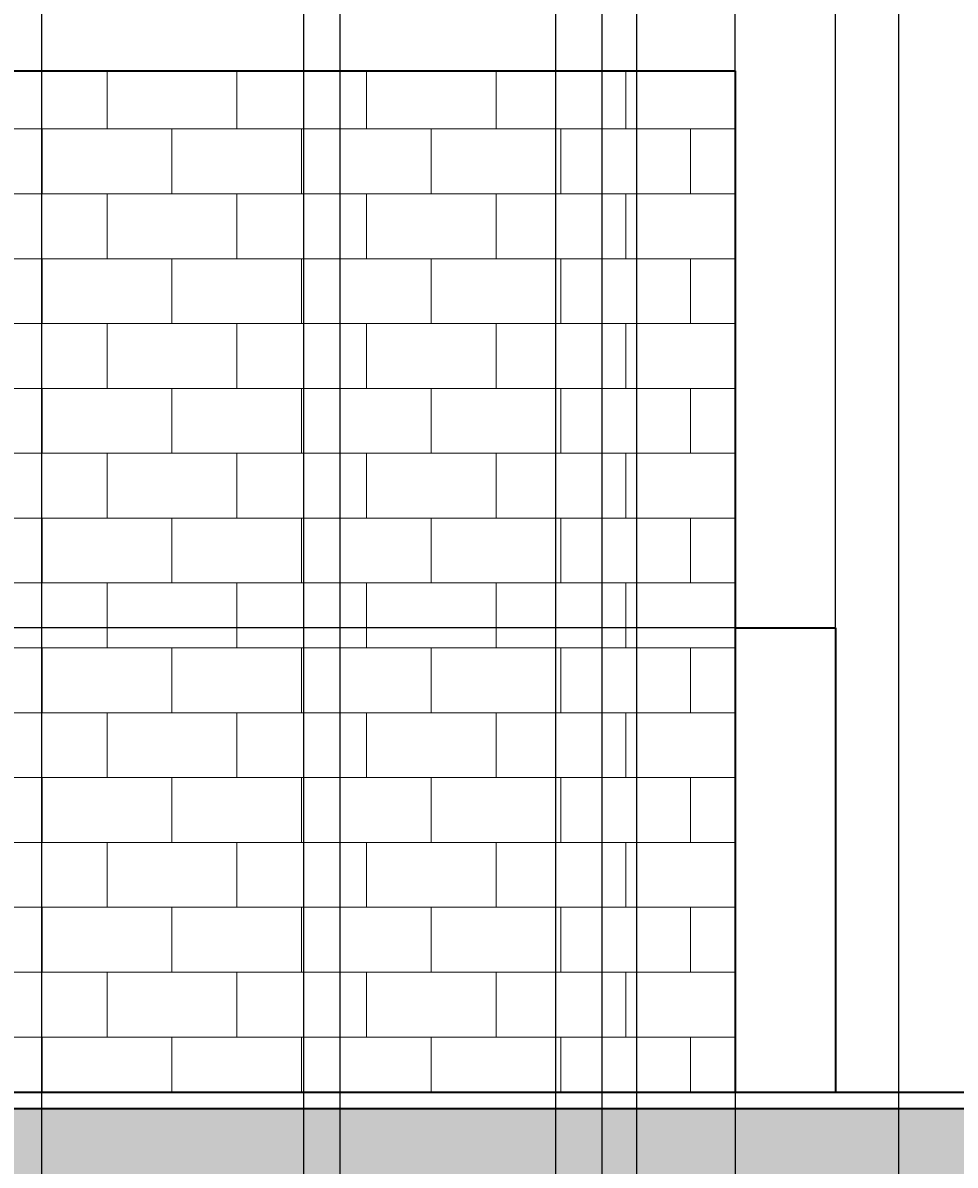
# Model space of a CAD drawing. Units: inches. Extents: x -5 to 714, y 84 to 644.
# Tile 12 of 20: x 342 to 457, y 336 to 477. Entities that reach past the tile are written whole.
import ezdxf

# ---------------------------------------------------------------- set-up
doc = ezdxf.new("R2010")
doc.units = ezdxf.units.IN
doc.header["$MEASUREMENT"] = 0
for name, color, linetype, lineweight in [('A-ANNO-DIMS', 2, 'Continuous', 18), ('A-ELEV', 7, 'Continuous', 35), ('A-ELEV-PATT', 8, 'Continuous', 13)]:
    doc.layers.add(name, color=color, linetype=linetype, lineweight=lineweight)
doc.styles.get("Standard").update_dxf_attribs({"font": 'arial.ttf'})
doc.dimstyles.get("Standard").update_dxf_attribs({"dimtxt": 0.9375, "dimasz": 0.18, "dimexe": 0.18, "dimexo": 0.0625, "dimgap": 0.09, "dimtad": 0, "dimtih": 1, "dimtoh": 1, "dimdec": 4, "dimzin": 0, "dimdsep": 46, "dimlunit": 4, "dimtxsty": 'Standard', "dimcen": 0.09, "dimadec": 0, "dimazin": 0, "dimtfac": 1, "dimtdec": 4, "dimtofl": 0, "dimtmove": 0, "dimatfit": 3, "dimfxl": 1, "dimtolj": 1, "dimtzin": 0, "dimarcsym": 0})

# ---------------------------------------------------------------- blocks, each defined once
blk = doc.blocks.new('*D27')
at = {"layer": 'A-ANNO-DIMS', "color": 0, "lineweight": -2, "transparency": 16777216}
for p, q in [((429.45, 402.48), (-2.74, 402.48)), ((-2.56, 402.3), (-2.56, 374.41)), ((-2.56, 345.37), (-2.56, 373.27)), ((429.45, 345.19), (-2.74, 345.19))]:
    blk.add_line(p, q, dxfattribs=at)
at = {"layer": 'A-ANNO-DIMS', "color": 0, "transparency": 16777216}
for points in [[(-2.59, 402.3), (-2.53, 402.3), (-2.56, 402.48)], [(-2.59, 345.37), (-2.53, 345.37), (-2.56, 345.19)]]:
    blk.add_solid(points, dxfattribs=at)
at = {"layer": 'Defpoints', "color": 0, "transparency": 16777216}
for p in [(-2.56, 402.48), (429.51, 402.48), (429.51, 345.19)]:
    blk.add_point(p, dxfattribs=at)
at = {"layer": 'A-ANNO-DIMS', "color": 0, "transparency": 16777216, "insert": (-2.56, 373.84), "char_height": 0.938, "attachment_point": 5}
blk.add_mtext('\\A1;57.29', dxfattribs=at)
blk = doc.blocks.new('*D29')
at = {"layer": 'A-ANNO-DIMS', "color": 0, "lineweight": -2, "transparency": 16777216}
for p, q in [((135.73, 471.11), (135.73, 84.31)), ((429.51, 471.11), (429.51, 84.31)), ((135.91, 84.49), (280.94, 84.49)), ((429.33, 84.49), (284.3, 84.49))]:
    blk.add_line(p, q, dxfattribs=at)
at = {"layer": 'A-ANNO-DIMS', "color": 0, "transparency": 16777216}
for points in [[(135.91, 84.52), (135.91, 84.46), (135.73, 84.49)], [(429.33, 84.52), (429.33, 84.46), (429.51, 84.49)]]:
    blk.add_solid(points, dxfattribs=at)
at = {"layer": 'Defpoints', "color": 0, "transparency": 16777216}
for p in [(135.73, 471.17), (429.51, 471.17), (429.51, 84.49)]:
    blk.add_point(p, dxfattribs=at)
at = {"layer": 'A-ANNO-DIMS', "color": 0, "transparency": 16777216, "insert": (282.62, 84.49), "char_height": 0.938, "attachment_point": 5}
blk.add_mtext('\\A1;293.8', dxfattribs=at)
blk = doc.blocks.new('*D30')
at = {"layer": 'A-ANNO-DIMS', "color": 0, "lineweight": -2, "transparency": 16777216}
for p, q in [((429.51, 402.54), (429.51, 643.61)), ((429.69, 643.43), (433.71, 643.43)), ((441.71, 643.43), (437.69, 643.43)), ((441.89, 402.54), (441.89, 643.61))]:
    blk.add_line(p, q, dxfattribs=at)
at = {"layer": 'A-ANNO-DIMS', "color": 0, "transparency": 16777216}
for points in [[(429.69, 643.46), (429.69, 643.4), (429.51, 643.43)], [(441.71, 643.46), (441.71, 643.4), (441.89, 643.43)]]:
    blk.add_solid(points, dxfattribs=at)
at = {"layer": 'Defpoints', "color": 0, "transparency": 16777216}
for p in [(441.89, 643.43), (429.51, 402.48), (441.89, 402.48)]:
    blk.add_point(p, dxfattribs=at)
at = {"layer": 'A-ANNO-DIMS', "color": 0, "transparency": 16777216, "insert": (435.7, 643.43), "char_height": 0.938, "attachment_point": 5}
blk.add_mtext('\\A1;12.378', dxfattribs=at)
blk = doc.blocks.new('*D54')
at = {"layer": 'A-ANNO-DIMS', "color": 0, "lineweight": -2, "transparency": 16777216}
for p, q in [((259.07, 315.16), (259.07, 643.61)), ((259.25, 643.43), (424.21, 643.43)), ((593.25, 643.43), (428.28, 643.43)), ((593.43, 315.16), (593.43, 643.61))]:
    blk.add_line(p, q, dxfattribs=at)
at = {"layer": 'A-ANNO-DIMS', "color": 0, "transparency": 16777216}
for points in [[(259.25, 643.46), (259.25, 643.4), (259.07, 643.43)], [(593.25, 643.46), (593.25, 643.4), (593.43, 643.43)]]:
    blk.add_solid(points, dxfattribs=at)
at = {"layer": 'Defpoints', "color": 0, "transparency": 16777216}
for p in [(593.43, 643.43), (259.07, 315.1), (593.43, 315.1)]:
    blk.add_point(p, dxfattribs=at)
at = {"layer": 'A-ANNO-DIMS', "color": 0, "transparency": 16777216, "insert": (426.25, 643.43), "char_height": 0.938, "attachment_point": 5}
blk.add_mtext('\\A1;334.36', dxfattribs=at)
blk = doc.blocks.new('*D61')
at = {"layer": 'A-ANNO-DIMS', "color": 0, "lineweight": -2, "transparency": 16777216}
for p, q in [((325.83, 266.06), (325.83, 643.61)), ((326.01, 643.43), (364.93, 643.43)), ((407.2, 643.43), (368.28, 643.43)), ((407.38, 266.06), (407.38, 643.61))]:
    blk.add_line(p, q, dxfattribs=at)
at = {"layer": 'A-ANNO-DIMS', "color": 0, "transparency": 16777216}
for points in [[(326.01, 643.46), (326.01, 643.4), (325.83, 643.43)], [(407.2, 643.46), (407.2, 643.4), (407.38, 643.43)]]:
    blk.add_solid(points, dxfattribs=at)
at = {"layer": 'Defpoints', "color": 0, "transparency": 16777216}
for p in [(407.38, 643.43), (325.83, 266), (407.38, 266)]:
    blk.add_point(p, dxfattribs=at)
at = {"layer": 'A-ANNO-DIMS', "color": 0, "transparency": 16777216, "insert": (366.61, 643.43), "char_height": 0.938, "attachment_point": 5}
blk.add_mtext('\\A1;81.55', dxfattribs=at)
blk = doc.blocks.new('*D62')
at = {"layer": 'A-ANNO-DIMS', "color": 0, "lineweight": -2, "transparency": 16777216}
for p, q in [((407.38, 266.06), (407.38, 643.61)), ((407.56, 643.43), (449.27, 643.43)), ((493.6, 643.43), (451.89, 643.43)), ((493.78, 266.06), (493.78, 643.61))]:
    blk.add_line(p, q, dxfattribs=at)
at = {"layer": 'A-ANNO-DIMS', "color": 0, "transparency": 16777216}
for points in [[(407.56, 643.46), (407.56, 643.4), (407.38, 643.43)], [(493.6, 643.46), (493.6, 643.4), (493.78, 643.43)]]:
    blk.add_solid(points, dxfattribs=at)
at = {"layer": 'Defpoints', "color": 0, "transparency": 16777216}
for p in [(493.78, 643.43), (407.38, 266), (493.78, 266)]:
    blk.add_point(p, dxfattribs=at)
at = {"layer": 'A-ANNO-DIMS', "color": 0, "transparency": 16777216, "insert": (450.58, 643.43), "char_height": 0.938, "attachment_point": 5}
blk.add_mtext('\\A1;86.4', dxfattribs=at)
blk = doc.blocks.new('*D84')
at = {"layer": 'A-ANNO-DIMS', "color": 0, "lineweight": -2, "transparency": 16777216}
for p, q in [((343.97, 144.93), (343.97, 643.61)), ((344.15, 643.43), (358.54, 643.43)), ((376.1, 643.43), (361.71, 643.43)), ((376.28, 144.93), (376.28, 643.61))]:
    blk.add_line(p, q, dxfattribs=at)
at = {"layer": 'A-ANNO-DIMS', "color": 0, "transparency": 16777216}
for points in [[(344.15, 643.46), (344.15, 643.4), (343.97, 643.43)], [(376.1, 643.46), (376.1, 643.4), (376.28, 643.43)]]:
    blk.add_solid(points, dxfattribs=at)
at = {"layer": 'Defpoints', "color": 0, "transparency": 16777216}
for p in [(376.28, 643.43), (343.97, 144.86), (376.28, 144.86)]:
    blk.add_point(p, dxfattribs=at)
at = {"layer": 'A-ANNO-DIMS', "color": 0, "transparency": 16777216, "insert": (360.13, 643.43), "char_height": 0.938, "attachment_point": 5}
blk.add_mtext('\\A1;32.31', dxfattribs=at)
blk = doc.blocks.new('*D85')
at = {"layer": 'A-ANNO-DIMS', "color": 0, "lineweight": -2, "transparency": 16777216}
for p, q in [((380.78, 144.93), (380.78, 643.61)), ((380.96, 643.43), (395.35, 643.43)), ((412.91, 643.43), (398.51, 643.43)), ((413.09, 144.93), (413.09, 643.61))]:
    blk.add_line(p, q, dxfattribs=at)
at = {"layer": 'A-ANNO-DIMS', "color": 0, "transparency": 16777216}
for points in [[(380.96, 643.46), (380.96, 643.4), (380.78, 643.43)], [(412.91, 643.46), (412.91, 643.4), (413.09, 643.43)]]:
    blk.add_solid(points, dxfattribs=at)
at = {"layer": 'Defpoints', "color": 0, "transparency": 16777216}
for p in [(413.09, 643.43), (380.78, 144.86), (413.09, 144.86)]:
    blk.add_point(p, dxfattribs=at)
at = {"layer": 'A-ANNO-DIMS', "color": 0, "transparency": 16777216, "insert": (396.93, 643.43), "char_height": 0.938, "attachment_point": 5}
blk.add_mtext('\\A1;32.31', dxfattribs=at)
blk = doc.blocks.new('*D86')
at = {"layer": 'A-ANNO-DIMS', "color": 0, "lineweight": -2, "transparency": 16777216}
for p, q in [((417.38, 144.93), (417.38, 643.61)), ((417.56, 643.43), (431.96, 643.43)), ((449.51, 643.43), (435.12, 643.43)), ((449.69, 144.93), (449.69, 643.61))]:
    blk.add_line(p, q, dxfattribs=at)
at = {"layer": 'A-ANNO-DIMS', "color": 0, "transparency": 16777216}
for points in [[(417.56, 643.46), (417.56, 643.4), (417.38, 643.43)], [(449.51, 643.46), (449.51, 643.4), (449.69, 643.43)]]:
    blk.add_solid(points, dxfattribs=at)
at = {"layer": 'Defpoints', "color": 0, "transparency": 16777216}
for p in [(449.69, 643.43), (417.38, 144.86), (449.69, 144.86)]:
    blk.add_point(p, dxfattribs=at)
at = {"layer": 'A-ANNO-DIMS', "color": 0, "transparency": 16777216, "insert": (433.54, 643.43), "char_height": 0.938, "attachment_point": 5}
blk.add_mtext('\\A1;32.31', dxfattribs=at)

msp = doc.modelspace()

# ---------------------------------------------------------------- hatches: boundary and pattern name
at = {"layer": 'A-ELEV-PATT', "transparency": 33554687}
h = msp.add_hatch(dxfattribs=at)
h.set_pattern_fill('AR-B816', color=256)
h.paths.add_polyline_path([(429.5094, 471.1709), (412.7784, 471.1709), (229.3575, 471.1709), (135.7303, 471.1709), (135.7303, 345.1928), (237.2654, 345.1928), (237.2654, 417.0908), (224.6446, 417.0908), (224.6446, 426.4485), (302.5023, 426.4485), (302.5023, 417.0908), (289.8815, 417.0908), (289.8815, 345.1928), (429.5094, 345.1928)])
h = msp.add_hatch(color=256, dxfattribs=at)
h.dxf.hatch_style = 1
h.paths.add_polyline_path([(584.2229, 343.1928), (259.0665, 343.1928), (259.0665, 315.0968), (584.2229, 315.0968)])
h.paths.add_polyline_path([(352.9482, 258.2864), (332.0052, 258.2864), (332.0052, 201.1928), (352.9482, 201.1928)])
h.paths.add_polyline_path([(378.5957, 258.2864), (357.6527, 258.2864), (357.6527, 201.1928), (378.5957, 201.1928)])
h.paths.add_polyline_path([(403.4391, 258.2864), (382.4961, 258.2864), (382.4961, 201.1928), (403.4391, 201.1928)])
h.paths.add_polyline_path([(339.2672, 197.3754), (332.0052, 197.3754), (332.0052, 191.3028), (339.2672, 191.3028)])
h.paths.add_polyline_path([(352.9482, 197.3754), (343.9704, 197.3754), (343.9704, 191.3028), (352.9482, 191.3028)])
h.paths.add_polyline_path([(352.9482, 189.3028), (343.9704, 189.3028), (343.9704, 184.8307), (352.9482, 184.8307)])
h.paths.add_polyline_path([(339.2672, 189.3028), (332.0052, 189.3028), (332.0052, 184.8307), (339.2672, 184.8307)])
h.paths.add_polyline_path([(339.2672, 182.8307), (332.0052, 182.8307), (332.0052, 177.6504), (339.2672, 177.6504)])
h.paths.add_polyline_path([(352.9482, 182.8307), (343.9704, 182.8307), (343.9704, 177.6504), (352.9482, 177.6504)])
h.paths.add_polyline_path([(352.9482, 175.6504), (343.9704, 175.6504), (343.9704, 173.6169), (352.9482, 173.6169)])
h.paths.add_polyline_path([(339.2672, 175.6504), (332.0052, 175.6504), (332.0052, 173.6169), (339.2672, 173.6169)])
h.paths.add_polyline_path([(376.2796, 175.6504), (357.6527, 175.6504), (357.6527, 173.6169), (376.2796, 173.6169)])
h.paths.add_polyline_path([(376.2796, 182.8307), (357.6527, 182.8307), (357.6527, 177.6504), (376.2796, 177.6504)])
h.paths.add_polyline_path([(376.2796, 189.3028), (357.6527, 189.3028), (357.6527, 184.8307), (376.2796, 184.8307)])
h.paths.add_polyline_path([(376.2796, 197.3754), (357.6527, 197.3754), (357.6527, 191.3028), (376.2796, 191.3028)])
h.paths.add_polyline_path([(403.4391, 197.3754), (382.4961, 197.3754), (382.4961, 191.3028), (403.4391, 191.3028)])
h.paths.add_polyline_path([(403.4391, 189.3028), (382.4961, 189.3028), (382.4961, 184.8307), (403.4391, 184.8307)])
h.paths.add_polyline_path([(403.4391, 182.8307), (382.4961, 182.8307), (382.4961, 177.6504), (403.4391, 177.6504)])
h.paths.add_polyline_path([(403.4391, 175.6504), (382.4961, 175.6504), (382.4961, 173.6169), (403.4391, 173.6169)])

# ---------------------------------------------------------------- linework, layer by layer
at = {"layer": 'A-ELEV'}
for p, q in [((229.3575, 471.1709), (412.7784, 471.1709)), ((412.7784, 471.1709), (429.5094, 471.1709)), ((429.5094, 471.1709), (429.5094, 345.1928)), ((429.5094, 402.4806), (441.8872, 402.4806)), ((441.8872, 402.4806), (441.8872, 345.1928)), ((67.9893, 345.1928), (587.5794, 345.1928)), ((259.0665, 343.1928), (584.2229, 343.1928))]:
    msp.add_line(p, q, dxfattribs=at)

# ---------------------------------------------------------------- dimensions: what is measured, and where the dimension line sits
at = {"layer": 'A-ANNO-DIMS'}
for base, p1, p2, override, picture, middle in [((593.428, 643.4276), (259.0665, 315.0968), (593.428, 315.0968), {"dimdec": 2, "dimlfac": 1, "dimrnd": 0, "dimzin": 0, "dimdsep": 46, "dimlunit": 2}, '*D54', (426.2472, 643.4276)), ((407.3813, 643.4276), (325.8305, 266.0021), (407.3813, 266.0021), {"dimdec": 2, "dimlfac": 1, "dimrnd": 0, "dimzin": 0, "dimdsep": 46, "dimlunit": 2}, '*D61', (366.6059, 643.4276)), ((376.2796, 643.4276), (343.9704, 144.8639), (376.2796, 144.8639), {"dimdec": 2, "dimlfac": 1, "dimrnd": 0, "dimzin": 0, "dimdsep": 46, "dimlunit": 2}, '*D84', (360.125, 643.4276)), ((413.0876, 643.4276), (380.7784, 144.8639), (413.0876, 144.8639), {"dimdec": 2, "dimlfac": 1, "dimrnd": 0, "dimzin": 0, "dimdsep": 46, "dimlunit": 2}, '*D85', (396.933, 643.4276)), ((493.7771, 643.4276), (407.3813, 266.0021), (493.7771, 266.0021), {"dimdec": 1, "dimlfac": 1, "dimrnd": 0, "dimzin": 0, "dimdsep": 46, "dimlunit": 2}, '*D62', (450.5792, 643.4276)), ((449.6911, 643.4276), (417.3818, 144.8639), (449.6911, 144.8639), {"dimdec": 2, "dimlfac": 1, "dimrnd": 0, "dimzin": 0, "dimdsep": 46, "dimlunit": 2}, '*D86', (433.5365, 643.4276)), ((441.8872, 643.4276), (429.5094, 402.4806), (441.8872, 402.4806), {"dimdec": 3, "dimlfac": 1, "dimrnd": 0, "dimzin": 0, "dimdsep": 46, "dimlunit": 2}, '*D30', (435.6983, 643.4276)), ((429.5094, 84.4928), (135.7303, 471.1709), (429.5094, 471.1709), {"dimdec": 1, "dimlfac": 1, "dimrnd": 0, "dimzin": 0, "dimdsep": 46, "dimlunit": 2}, '*D29', (282.6198, 84.4928))]:
    dim = msp.add_linear_dim(base=base, p1=p1, p2=p2, dimstyle='Standard', override=override, dxfattribs=at)
    dim.commit()
    dim.dimension.update_dxf_attribs({"geometry": picture, "text_midpoint": middle})
dim = msp.add_linear_dim(base=(-2.5605, 402.4806), p1=(429.5094, 345.1928), p2=(429.5094, 402.4806), angle=90, dimstyle='Standard', override={"dimdec": 2, "dimlfac": 1, "dimrnd": 0, "dimzin": 0, "dimdsep": 46, "dimlunit": 2}, dxfattribs=at)
dim.commit()
dim.dimension.update_dxf_attribs({"geometry": '*D27', "text_midpoint": (-2.5605, 373.8367)})

doc.saveas('drawing.dxf')
